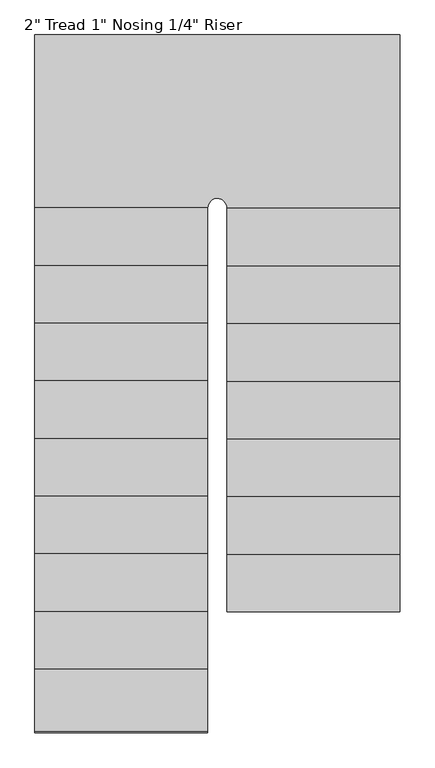
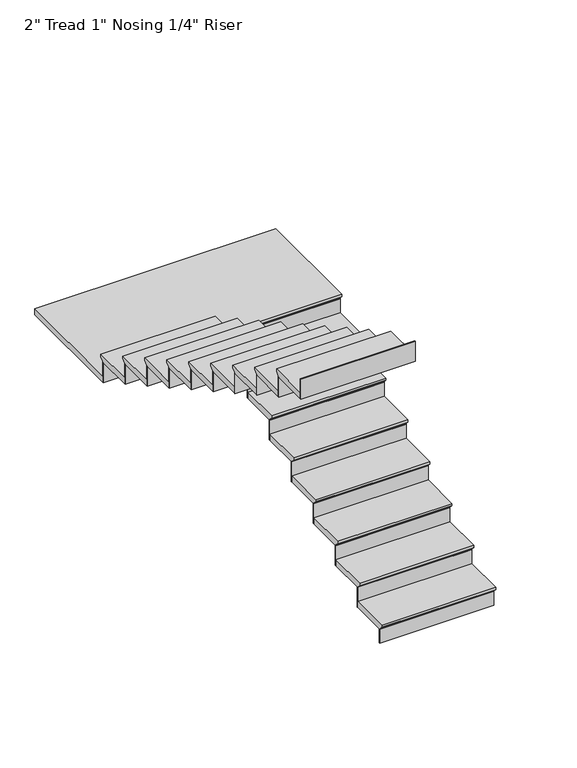
"""IFC4 building model written with IfcOpenShell, lengths in millimetres: stair flight geometry."""

from ifc_helpers import new_model, si_unit, frame, origin, place, context, project, spatial, polyline, circle_curve, ellipse_curve, faceted_brep, source, transform, mapped, element, save
from ifc_brep_helpers import plane_surface, revolved_surface, advanced_brep


def stair_flight_d4afe6aa(model_context):
    return source(origin(), model_context, "Body", "SolidModel", [
        faceted_brep([(-2547.8656154, 3686.6500875, 3198.2833333), (-2547.8656154, 3686.6500875, 3217.3333333), (-3462.2656154, 3686.6500875, 3217.3333333), (-3462.2656154, 3686.6500875, 3198.2833333), (-2547.8656154, 3712.0500875, 3172.8833333), (-3462.2656154, 3712.0500875, 3172.8833333), (-2547.8656154, 4016.8500875, 3217.3333333), (-3462.2656154, 4016.8500875, 3217.3333333), (-3462.2656154, 3712.0500875, 3166.5333333), (-3462.2656154, 4016.8500875, 3166.5333333), (-2547.8656154, 4016.8500875, 3166.5333333), (-2547.8656154, 3712.0500875, 3166.5333333)], [[[0, 1, 2, 3]], [[4, 0, 3, 5]], [[2, 1, 6, 7]], [[8, 9, 10, 11]], [[2, 7, 9, 8, 5, 3]], [[8, 11, 4, 5]], [[6, 1, 0, 4, 11, 10]], [[7, 6, 10, 9]]]),
        faceted_brep([(-2547.8656154, 3712.0500875, 3166.5333333), (-2547.8656154, 3712.0500875, 3048.0), (-2547.8656154, 3718.4000875, 3048.0), (-2547.8656154, 3718.4000875, 3166.5333333), (-3462.2656154, 3712.0500875, 3166.5333333), (-3462.2656154, 3718.4000875, 3166.5333333), (-3462.2656154, 3718.4000875, 3048.0), (-3462.2656154, 3712.0500875, 3048.0)], [[[0, 1, 2, 3]], [[4, 5, 6, 7]], [[1, 0, 4, 7]], [[2, 1, 7, 6]], [[3, 2, 6, 5]], [[0, 3, 5, 4]]]),
        faceted_brep([(-2547.8656154, 4016.8500875, 3335.8666667), (-2547.8656154, 4016.8500875, 3166.5333333), (-2547.8656154, 4023.2000875, 3166.5333333), (-2547.8656154, 4023.2000875, 3335.8666667), (-3462.2656154, 4016.8500875, 3335.8666667), (-3462.2656154, 4023.2000875, 3335.8666667), (-3462.2656154, 4023.2000875, 3166.5333333), (-3462.2656154, 4016.8500875, 3166.5333333)], [[[0, 1, 2, 3]], [[4, 5, 6, 7]], [[1, 0, 4, 7]], [[2, 1, 7, 6]], [[3, 2, 6, 5]], [[0, 3, 5, 4]]]),
        faceted_brep([(-3462.2656154, 3991.4500875, 3386.6666667), (-2547.8656154, 3991.4500875, 3386.6666667), (-2547.8656154, 4321.6500875, 3386.6666667), (-3462.2656154, 4321.6500875, 3386.6666667), (-3462.2656154, 4016.8500875, 3335.8666667), (-3462.2656154, 4321.6500875, 3335.8666667), (-2547.8656154, 4321.6500875, 3335.8666667), (-2547.8656154, 4016.8500875, 3335.8666667), (-3462.2656154, 4016.8500875, 3342.2166667), (-3462.2656154, 3991.4500875, 3367.6166667), (-2547.8656154, 4016.8500875, 3342.2166667), (-2547.8656154, 3991.4500875, 3367.6166667)], [[[0, 1, 2, 3]], [[4, 5, 6, 7]], [[0, 3, 5, 4, 8, 9]], [[4, 7, 10, 8]], [[2, 1, 11, 10, 7, 6]], [[3, 2, 6, 5]], [[11, 1, 0, 9]], [[10, 11, 9, 8]]]),
        faceted_brep([(-2547.8656154, 4321.6500875, 3505.2), (-2547.8656154, 4321.6500875, 3335.8666667), (-2547.8656154, 4328.0000875, 3335.8666667), (-2547.8656154, 4328.0000875, 3505.2), (-3462.2656154, 4321.6500875, 3505.2), (-3462.2656154, 4328.0000875, 3505.2), (-3462.2656154, 4328.0000875, 3335.8666667), (-3462.2656154, 4321.6500875, 3335.8666667)], [[[0, 1, 2, 3]], [[4, 5, 6, 7]], [[1, 0, 4, 7]], [[2, 1, 7, 6]], [[3, 2, 6, 5]], [[0, 3, 5, 4]]]),
        faceted_brep([(-3462.2656154, 4296.2500875, 3556.0), (-2547.8656154, 4296.2500875, 3556.0), (-2547.8656154, 4626.4500875, 3556.0), (-3462.2656154, 4626.4500875, 3556.0), (-3462.2656154, 4321.6500875, 3505.2), (-3462.2656154, 4626.4500875, 3505.2), (-2547.8656154, 4626.4500875, 3505.2), (-2547.8656154, 4321.6500875, 3505.2), (-3462.2656154, 4321.6500875, 3511.55), (-3462.2656154, 4296.2500875, 3536.95), (-2547.8656154, 4321.6500875, 3511.55), (-2547.8656154, 4296.2500875, 3536.95)], [[[0, 1, 2, 3]], [[4, 5, 6, 7]], [[0, 3, 5, 4, 8, 9]], [[4, 7, 10, 8]], [[2, 1, 11, 10, 7, 6]], [[3, 2, 6, 5]], [[11, 1, 0, 9]], [[10, 11, 9, 8]]]),
        faceted_brep([(-2547.8656154, 4626.4500875, 3674.5333333), (-2547.8656154, 4626.4500875, 3505.2), (-2547.8656154, 4632.8000875, 3505.2), (-2547.8656154, 4632.8000875, 3674.5333333), (-3462.2656154, 4626.4500875, 3674.5333333), (-3462.2656154, 4632.8000875, 3674.5333333), (-3462.2656154, 4632.8000875, 3505.2), (-3462.2656154, 4626.4500875, 3505.2)], [[[0, 1, 2, 3]], [[4, 5, 6, 7]], [[1, 0, 4, 7]], [[2, 1, 7, 6]], [[3, 2, 6, 5]], [[0, 3, 5, 4]]]),
        faceted_brep([(-3462.2656154, 4601.0500875, 3725.3333333), (-2547.8656154, 4601.0500875, 3725.3333333), (-2547.8656154, 4931.2500875, 3725.3333333), (-3462.2656154, 4931.2500875, 3725.3333333), (-3462.2656154, 4626.4500875, 3674.5333333), (-3462.2656154, 4931.2500875, 3674.5333333), (-2547.8656154, 4931.2500875, 3674.5333333), (-2547.8656154, 4626.4500875, 3674.5333333), (-3462.2656154, 4626.4500875, 3680.8833333), (-3462.2656154, 4601.0500875, 3706.2833333), (-2547.8656154, 4626.4500875, 3680.8833333), (-2547.8656154, 4601.0500875, 3706.2833333)], [[[0, 1, 2, 3]], [[4, 5, 6, 7]], [[0, 3, 5, 4, 8, 9]], [[4, 7, 10, 8]], [[2, 1, 11, 10, 7, 6]], [[3, 2, 6, 5]], [[11, 1, 0, 9]], [[10, 11, 9, 8]]]),
        faceted_brep([(-2547.8656154, 4931.2500875, 3843.8666667), (-2547.8656154, 4931.2500875, 3674.5333333), (-2547.8656154, 4937.6000875, 3674.5333333), (-2547.8656154, 4937.6000875, 3843.8666667), (-3462.2656154, 4931.2500875, 3843.8666667), (-3462.2656154, 4937.6000875, 3843.8666667), (-3462.2656154, 4937.6000875, 3674.5333333), (-3462.2656154, 4931.2500875, 3674.5333333)], [[[0, 1, 2, 3]], [[4, 5, 6, 7]], [[1, 0, 4, 7]], [[2, 1, 7, 6]], [[3, 2, 6, 5]], [[0, 3, 5, 4]]]),
        faceted_brep([(-3462.2656154, 4905.8500875, 3894.6666667), (-2547.8656154, 4905.8500875, 3894.6666667), (-2547.8656154, 5236.0500875, 3894.6666667), (-3462.2656154, 5236.0500875, 3894.6666667), (-3462.2656154, 4931.2500875, 3843.8666667), (-3462.2656154, 5236.0500875, 3843.8666667), (-2547.8656154, 5236.0500875, 3843.8666667), (-2547.8656154, 4931.2500875, 3843.8666667), (-3462.2656154, 4931.2500875, 3850.2166667), (-3462.2656154, 4905.8500875, 3875.6166667), (-2547.8656154, 4931.2500875, 3850.2166667), (-2547.8656154, 4905.8500875, 3875.6166667)], [[[0, 1, 2, 3]], [[4, 5, 6, 7]], [[0, 3, 5, 4, 8, 9]], [[4, 7, 10, 8]], [[2, 1, 11, 10, 7, 6]], [[3, 2, 6, 5]], [[11, 1, 0, 9]], [[10, 11, 9, 8]]]),
        faceted_brep([(-2547.8656154, 5236.0500875, 4013.2), (-2547.8656154, 5236.0500875, 3843.8666667), (-2547.8656154, 5242.4000875, 3843.8666667), (-2547.8656154, 5242.4000875, 4013.2), (-3462.2656154, 5236.0500875, 4013.2), (-3462.2656154, 5242.4000875, 4013.2), (-3462.2656154, 5242.4000875, 3843.8666667), (-3462.2656154, 5236.0500875, 3843.8666667)], [[[0, 1, 2, 3]], [[4, 5, 6, 7]], [[1, 0, 4, 7]], [[2, 1, 7, 6]], [[3, 2, 6, 5]], [[0, 3, 5, 4]]]),
        faceted_brep([(-3462.2656154, 5210.6500875, 4064.0), (-2547.8656154, 5210.6500875, 4064.0), (-2547.8656154, 5540.8500875, 4064.0), (-3462.2656154, 5540.8500875, 4064.0), (-3462.2656154, 5236.0500875, 4013.2), (-3462.2656154, 5540.8500875, 4013.2), (-2547.8656154, 5540.8500875, 4013.2), (-2547.8656154, 5236.0500875, 4013.2), (-3462.2656154, 5236.0500875, 4019.55), (-3462.2656154, 5210.6500875, 4044.95), (-2547.8656154, 5236.0500875, 4019.55), (-2547.8656154, 5210.6500875, 4044.95)], [[[0, 1, 2, 3]], [[4, 5, 6, 7]], [[0, 3, 5, 4, 8, 9]], [[4, 7, 10, 8]], [[2, 1, 11, 10, 7, 6]], [[3, 2, 6, 5]], [[11, 1, 0, 9]], [[10, 11, 9, 8]]]),
        faceted_brep([(-2547.8656154, 5540.8500875, 4182.5333333), (-2547.8656154, 5540.8500875, 4013.2), (-2547.8656154, 5547.2000875, 4013.2), (-2547.8656154, 5547.2000875, 4182.5333333), (-3462.2656154, 5540.8500875, 4182.5333333), (-3462.2656154, 5547.2000875, 4182.5333333), (-3462.2656154, 5547.2000875, 4013.2), (-3462.2656154, 5540.8500875, 4013.2)], [[[0, 1, 2, 3]], [[4, 5, 6, 7]], [[1, 0, 4, 7]], [[2, 1, 7, 6]], [[3, 2, 6, 5]], [[0, 3, 5, 4]]]),
        faceted_brep([(-3462.2656154, 5515.4500875, 4233.3333333), (-2547.8656154, 5515.4500875, 4233.3333333), (-2547.8656154, 5845.6500875, 4233.3333333), (-3462.2656154, 5845.6500875, 4233.3333333), (-3462.2656154, 5540.8500875, 4182.5333333), (-3462.2656154, 5845.6500875, 4182.5333333), (-2547.8656154, 5845.6500875, 4182.5333333), (-2547.8656154, 5540.8500875, 4182.5333333), (-3462.2656154, 5540.8500875, 4188.8833333), (-3462.2656154, 5515.4500875, 4214.2833333), (-2547.8656154, 5540.8500875, 4188.8833333), (-2547.8656154, 5515.4500875, 4214.2833333)], [[[0, 1, 2, 3]], [[4, 5, 6, 7]], [[0, 3, 5, 4, 8, 9]], [[4, 7, 10, 8]], [[2, 1, 11, 10, 7, 6]], [[3, 2, 6, 5]], [[11, 1, 0, 9]], [[10, 11, 9, 8]]]),
        advanced_brep(
        [(-2547.8656154, 5845.6500875, 4351.8666667), (-2547.8656154, 5845.6500875, 4182.5333333), (-2547.8656154, 5852.0000875, 4182.5333333), (-2547.8656154, 5852.0000875, 4351.8666667), (-3469.0715249, 5845.6500875, 4351.8666667), (-3473.4098781, 5852.0000875, 4351.8666667), (-3473.4098781, 5852.0000875, 4182.5333333), (-3469.0715249, 5845.6500875, 4182.5333333)],
        [
            (0, 1),
            (1, 2),
            (2, 3),
            (3, 0),
            (4, 5, circle_curve(frame((-3513.0656154, 5820.2500875, 4351.8666667), z_axis=(0.0, 0.0, 1.0), x_axis=(1.0, 0.0, 0.0)), 50.8)),
            (5, 6),
            (6, 7, circle_curve(frame((-3513.0656154, 5820.2500875, 4182.5333333), z_axis=(0.0, 0.0, -1.0), x_axis=(1.0, 0.0, 0.0)), 50.8)),
            (7, 4),
            (0, 4),
            (7, 1),
            (6, 2),
            (5, 3),
        ],
        [
            plane_surface(frame((-2547.8656154, 5845.6500875, 4402.6666667), z_axis=(1.0, 0.0, 0.0), x_axis=(0.0, 1.0, 0.0))),
            revolved_surface(polyline([(-3462.2656153999997, 5820.2500875, 4182.5333333), (-3462.2656153999997, 5820.2500875, 4351.8666667)]), (-3513.0656154, 5820.2500875, 4351.8666667), (0.0, 0.0, -1.0)),
            plane_surface(frame((-2547.8656154, 5845.6500875, 4351.8666667), z_axis=(0.0, -1.0, 0.0), x_axis=(-1.0, 0.0, 0.0))),
            plane_surface(frame((-2547.8656154, 5845.6500875, 4182.5333333), z_axis=(0.0, 0.0, -1.0), x_axis=(-1.0, 0.0, 0.0))),
            plane_surface(frame((-2547.8656154, 5852.0000875, 4182.5333333), z_axis=(0.0, 1.0, 0.0), x_axis=(-1.0, 0.0, 0.0))),
            plane_surface(frame((-2547.8656154, 5852.0000875, 4351.8666667), z_axis=(0.0, 0.0, 1.0), x_axis=(-1.0, 0.0, 0.0))),
        ],
        [
            (0, [[1, 2, 3, 4]]),
            (1, [[5, 6, 7, 8]]),
            (2, [[-1, 9, -8, 10]]),
            (3, [[-2, -10, -7, 11]]),
            (4, [[-3, -11, -6, 12]]),
            (5, [[-4, -12, -5, -9]]),
        ],
    ),
        advanced_brep(
        [(-3563.8656154, 5794.8500875, 4402.6666667), (-3563.8656154, 5820.2500875, 4402.6666667), (-3469.0715249, 5845.6500875, 4402.6666667), (-3462.2656154, 5820.2500875, 4402.6666667), (-2547.8656154, 5820.2500875, 4402.6666667), (-2547.8656154, 6734.6500875, 4402.6666667), (-4478.2656154, 6734.6500875, 4402.6666667), (-4478.2656154, 5794.8500875, 4402.6666667), (-3563.8656154, 5820.2500875, 4351.8666667), (-3563.8656154, 5794.8500875, 4351.8666667), (-4478.2656154, 5794.8500875, 4351.8666667), (-4478.2656154, 6734.6500875, 4351.8666667), (-2547.8656154, 6734.6500875, 4351.8666667), (-2547.8656154, 5845.6500875, 4351.8666667), (-3469.0715249, 5845.6500875, 4351.8666667), (-3469.0715249, 5845.6500875, 4358.2166667), (-2547.8656154, 5845.6500875, 4358.2166667), (-2547.8656154, 5820.2500875, 4383.6166667), (-3462.2656154, 5820.2500875, 4383.6166667)],
        [
            (0, 1),
            (1, 2, circle_curve(frame((-3513.0656154, 5820.2500875, 4402.6666667), z_axis=(0.0, 0.0, -1.0), x_axis=(1.0, 0.0, 0.0)), 50.8)),
            (2, 3, circle_curve(frame((-3513.0656154, 5820.2500875, 4402.6666667), z_axis=(0.0, 0.0, -1.0), x_axis=(1.0, 0.0, 0.0)), 50.8)),
            (3, 4),
            (4, 5),
            (5, 6),
            (6, 7),
            (7, 0),
            (8, 9),
            (9, 10),
            (10, 11),
            (11, 12),
            (12, 13),
            (13, 14),
            (14, 8, circle_curve(frame((-3513.0656154, 5820.2500875, 4351.8666667), z_axis=(0.0, 0.0, 1.0), x_axis=(1.0, 0.0, 0.0)), 50.8)),
            (0, 9),
            (8, 1),
            (14, 15),
            (15, 2),
            (13, 16),
            (16, 15),
            (4, 17),
            (17, 16),
            (12, 5),
            (11, 6),
            (10, 7),
            (18, 3),
            (15, 18, ellipse_curve(frame((-3513.0656154, 5820.2500875, 4383.6166667), z_axis=(0.0, -0.7071067811865489, -0.7071067811865461), x_axis=(0.0, 0.7071067811865461, -0.7071067811865489)), 71.842049, 50.8)),
            (18, 17),
        ],
        [
            plane_surface(frame((-3563.8656154, 5820.2500875, 4402.6666667), z_axis=(0.0, 0.0, 1.0), x_axis=(0.0, 1.0, 0.0))),
            plane_surface(frame((-3563.8656154, 5820.2500875, 4351.8666667), z_axis=(0.0, 0.0, -1.0), x_axis=(0.0, -1.0, 0.0))),
            plane_surface(frame((-3563.8656154, 5794.8500875, 4402.6666667), z_axis=(1.0, 0.0, 0.0), x_axis=(0.0, 0.0, -1.0))),
            revolved_surface(polyline([(-3462.2656153999997, 5820.2500875, 4351.8666667), (-3462.2656153999997, 5820.2500875, 4402.6666667)]), (-3513.0656154, 5820.2500875, 4351.8666667), (0.0, 0.0, -1.0)),
            plane_surface(frame((-3469.0715249, 5845.6500875, 4402.6666667), z_axis=(0.0, -1.0, 0.0), x_axis=(0.0, 0.0, -1.0))),
            plane_surface(frame((-2547.8656154, 5845.6500875, 4402.6666667), z_axis=(1.0, 0.0, 0.0), x_axis=(0.0, 0.0, -1.0))),
            plane_surface(frame((-2547.8656154, 6734.6500875, 4402.6666667), z_axis=(0.0, 1.0, 0.0), x_axis=(0.0, 0.0, -1.0))),
            plane_surface(frame((-4478.2656154, 6734.6500875, 4402.6666667), z_axis=(-1.0, 0.0, 0.0), x_axis=(0.0, 0.0, -1.0))),
            plane_surface(frame((-4478.2656154, 5794.8500875, 4402.6666667), z_axis=(0.0, -1.0, 0.0), x_axis=(0.0, 0.0, -1.0))),
            revolved_surface(polyline([(-3462.2656153999997, 5820.2500875, 4332.816666677763), (-3462.2656153999997, 5820.2500875, 4434.416666722236)]), (-3513.0656154, 5820.2500875, 4351.8666667), (0.0, 0.0, -1.0)),
            plane_surface(frame((-2547.8656154, 5820.2500875, 4402.6666667), z_axis=(0.0, -1.0, 0.0), x_axis=(-1.0, 0.0, 0.0))),
            plane_surface(frame((-2547.8656154, 5820.2500875, 4383.6166667), z_axis=(0.0, -0.7071067811865489, -0.7071067811865461), x_axis=(-1.0, 0.0, 0.0))),
        ],
        [
            (0, [[1, 2, 3, 4, 5, 6, 7, 8]]),
            (1, [[9, 10, 11, 12, 13, 14, 15]]),
            (2, [[-1, 16, -9, 17]]),
            (3, [[-2, -17, -15, 18, 19]]),
            (4, [[-14, 20, 21, -18]]),
            (5, [[-5, 22, 23, -20, -13, 24]]),
            (6, [[-6, -24, -12, 25]]),
            (7, [[-7, -25, -11, 26]]),
            (8, [[-8, -26, -10, -16]]),
            (9, [[27, -3, -19, 28]]),
            (10, [[-22, -4, -27, 29]]),
            (11, [[-23, -29, -28, -21]]),
        ],
    ),
        faceted_brep([(-4478.2656154, 5794.8500875, 4521.2), (-4478.2656154, 5794.8500875, 4351.8666667), (-4478.2656154, 5788.5000875, 4351.8666667), (-4478.2656154, 5788.5000875, 4521.2), (-3563.8656154, 5794.8500875, 4521.2), (-3563.8656154, 5788.5000875, 4521.2), (-3563.8656154, 5788.5000875, 4351.8666667), (-3563.8656154, 5794.8500875, 4351.8666667)], [[[0, 1, 2, 3]], [[4, 5, 6, 7]], [[1, 0, 4, 7]], [[2, 1, 7, 6]], [[3, 2, 6, 5]], [[0, 3, 5, 4]]]),
        faceted_brep([(-3563.8656154, 5820.2500875, 4572.0), (-4478.2656154, 5820.2500875, 4572.0), (-4478.2656154, 5490.0500875, 4572.0), (-3563.8656154, 5490.0500875, 4572.0), (-3563.8656154, 5794.8500875, 4521.2), (-3563.8656154, 5490.0500875, 4521.2), (-4478.2656154, 5490.0500875, 4521.2), (-4478.2656154, 5794.8500875, 4521.2), (-3563.8656154, 5794.8500875, 4527.55), (-3563.8656154, 5820.2500875, 4552.95), (-4478.2656154, 5794.8500875, 4527.55), (-4478.2656154, 5820.2500875, 4552.95)], [[[0, 1, 2, 3]], [[4, 5, 6, 7]], [[0, 3, 5, 4, 8, 9]], [[4, 7, 10, 8]], [[2, 1, 11, 10, 7, 6]], [[3, 2, 6, 5]], [[11, 1, 0, 9]], [[10, 11, 9, 8]]]),
        faceted_brep([(-4478.2656154, 5490.0500875, 4690.5333333), (-4478.2656154, 5490.0500875, 4521.2), (-4478.2656154, 5483.7000875, 4521.2), (-4478.2656154, 5483.7000875, 4690.5333333), (-3563.8656154, 5490.0500875, 4690.5333333), (-3563.8656154, 5483.7000875, 4690.5333333), (-3563.8656154, 5483.7000875, 4521.2), (-3563.8656154, 5490.0500875, 4521.2)], [[[0, 1, 2, 3]], [[4, 5, 6, 7]], [[1, 0, 4, 7]], [[2, 1, 7, 6]], [[3, 2, 6, 5]], [[0, 3, 5, 4]]]),
        faceted_brep([(-3563.8656154, 5515.4500875, 4741.3333333), (-4478.2656154, 5515.4500875, 4741.3333333), (-4478.2656154, 5185.2500875, 4741.3333333), (-3563.8656154, 5185.2500875, 4741.3333333), (-3563.8656154, 5490.0500875, 4690.5333333), (-3563.8656154, 5185.2500875, 4690.5333333), (-4478.2656154, 5185.2500875, 4690.5333333), (-4478.2656154, 5490.0500875, 4690.5333333), (-3563.8656154, 5490.0500875, 4696.8833333), (-3563.8656154, 5515.4500875, 4722.2833333), (-4478.2656154, 5490.0500875, 4696.8833333), (-4478.2656154, 5515.4500875, 4722.2833333)], [[[0, 1, 2, 3]], [[4, 5, 6, 7]], [[0, 3, 5, 4, 8, 9]], [[4, 7, 10, 8]], [[2, 1, 11, 10, 7, 6]], [[3, 2, 6, 5]], [[11, 1, 0, 9]], [[10, 11, 9, 8]]]),
        faceted_brep([(-4478.2656154, 5185.2500875, 4859.8666667), (-4478.2656154, 5185.2500875, 4690.5333333), (-4478.2656154, 5178.9000875, 4690.5333333), (-4478.2656154, 5178.9000875, 4859.8666667), (-3563.8656154, 5185.2500875, 4859.8666667), (-3563.8656154, 5178.9000875, 4859.8666667), (-3563.8656154, 5178.9000875, 4690.5333333), (-3563.8656154, 5185.2500875, 4690.5333333)], [[[0, 1, 2, 3]], [[4, 5, 6, 7]], [[1, 0, 4, 7]], [[2, 1, 7, 6]], [[3, 2, 6, 5]], [[0, 3, 5, 4]]]),
        faceted_brep([(-3563.8656154, 5210.6500875, 4910.6666667), (-4478.2656154, 5210.6500875, 4910.6666667), (-4478.2656154, 4880.4500875, 4910.6666667), (-3563.8656154, 4880.4500875, 4910.6666667), (-3563.8656154, 5185.2500875, 4859.8666667), (-3563.8656154, 4880.4500875, 4859.8666667), (-4478.2656154, 4880.4500875, 4859.8666667), (-4478.2656154, 5185.2500875, 4859.8666667), (-3563.8656154, 5185.2500875, 4866.2166667), (-3563.8656154, 5210.6500875, 4891.6166667), (-4478.2656154, 5185.2500875, 4866.2166667), (-4478.2656154, 5210.6500875, 4891.6166667)], [[[0, 1, 2, 3]], [[4, 5, 6, 7]], [[0, 3, 5, 4, 8, 9]], [[4, 7, 10, 8]], [[2, 1, 11, 10, 7, 6]], [[3, 2, 6, 5]], [[11, 1, 0, 9]], [[10, 11, 9, 8]]]),
        faceted_brep([(-4478.2656154, 4880.4500875, 5029.2), (-4478.2656154, 4880.4500875, 4859.8666667), (-4478.2656154, 4874.1000875, 4859.8666667), (-4478.2656154, 4874.1000875, 5029.2), (-3563.8656154, 4880.4500875, 5029.2), (-3563.8656154, 4874.1000875, 5029.2), (-3563.8656154, 4874.1000875, 4859.8666667), (-3563.8656154, 4880.4500875, 4859.8666667)], [[[0, 1, 2, 3]], [[4, 5, 6, 7]], [[1, 0, 4, 7]], [[2, 1, 7, 6]], [[3, 2, 6, 5]], [[0, 3, 5, 4]]]),
        faceted_brep([(-3563.8656154, 4905.8500875, 5080.0), (-4478.2656154, 4905.8500875, 5080.0), (-4478.2656154, 4575.6500875, 5080.0), (-3563.8656154, 4575.6500875, 5080.0), (-3563.8656154, 4880.4500875, 5029.2), (-3563.8656154, 4575.6500875, 5029.2), (-4478.2656154, 4575.6500875, 5029.2), (-4478.2656154, 4880.4500875, 5029.2), (-3563.8656154, 4880.4500875, 5035.55), (-3563.8656154, 4905.8500875, 5060.95), (-4478.2656154, 4880.4500875, 5035.55), (-4478.2656154, 4905.8500875, 5060.95)], [[[0, 1, 2, 3]], [[4, 5, 6, 7]], [[0, 3, 5, 4, 8, 9]], [[4, 7, 10, 8]], [[2, 1, 11, 10, 7, 6]], [[3, 2, 6, 5]], [[11, 1, 0, 9]], [[10, 11, 9, 8]]]),
        faceted_brep([(-4478.2656154, 4575.6500875, 5198.5333333), (-4478.2656154, 4575.6500875, 5029.2), (-4478.2656154, 4569.3000875, 5029.2), (-4478.2656154, 4569.3000875, 5198.5333333), (-3563.8656154, 4575.6500875, 5198.5333333), (-3563.8656154, 4569.3000875, 5198.5333333), (-3563.8656154, 4569.3000875, 5029.2), (-3563.8656154, 4575.6500875, 5029.2)], [[[0, 1, 2, 3]], [[4, 5, 6, 7]], [[1, 0, 4, 7]], [[2, 1, 7, 6]], [[3, 2, 6, 5]], [[0, 3, 5, 4]]]),
        faceted_brep([(-3563.8656154, 4601.0500875, 5249.3333333), (-4478.2656154, 4601.0500875, 5249.3333333), (-4478.2656154, 4270.8500875, 5249.3333333), (-3563.8656154, 4270.8500875, 5249.3333333), (-3563.8656154, 4575.6500875, 5198.5333333), (-3563.8656154, 4270.8500875, 5198.5333333), (-4478.2656154, 4270.8500875, 5198.5333333), (-4478.2656154, 4575.6500875, 5198.5333333), (-3563.8656154, 4575.6500875, 5204.8833333), (-3563.8656154, 4601.0500875, 5230.2833333), (-4478.2656154, 4575.6500875, 5204.8833333), (-4478.2656154, 4601.0500875, 5230.2833333)], [[[0, 1, 2, 3]], [[4, 5, 6, 7]], [[0, 3, 5, 4, 8, 9]], [[4, 7, 10, 8]], [[2, 1, 11, 10, 7, 6]], [[3, 2, 6, 5]], [[11, 1, 0, 9]], [[10, 11, 9, 8]]]),
        faceted_brep([(-4478.2656154, 4270.8500875, 5367.8666667), (-4478.2656154, 4270.8500875, 5198.5333333), (-4478.2656154, 4264.5000875, 5198.5333333), (-4478.2656154, 4264.5000875, 5367.8666667), (-3563.8656154, 4270.8500875, 5367.8666667), (-3563.8656154, 4264.5000875, 5367.8666667), (-3563.8656154, 4264.5000875, 5198.5333333), (-3563.8656154, 4270.8500875, 5198.5333333)], [[[0, 1, 2, 3]], [[4, 5, 6, 7]], [[1, 0, 4, 7]], [[2, 1, 7, 6]], [[3, 2, 6, 5]], [[0, 3, 5, 4]]]),
        faceted_brep([(-3563.8656154, 4296.2500875, 5418.6666667), (-4478.2656154, 4296.2500875, 5418.6666667), (-4478.2656154, 3966.0500875, 5418.6666667), (-3563.8656154, 3966.0500875, 5418.6666667), (-3563.8656154, 4270.8500875, 5367.8666667), (-3563.8656154, 3966.0500875, 5367.8666667), (-4478.2656154, 3966.0500875, 5367.8666667), (-4478.2656154, 4270.8500875, 5367.8666667), (-3563.8656154, 4270.8500875, 5374.2166667), (-3563.8656154, 4296.2500875, 5399.6166667), (-4478.2656154, 4270.8500875, 5374.2166667), (-4478.2656154, 4296.2500875, 5399.6166667)], [[[0, 1, 2, 3]], [[4, 5, 6, 7]], [[0, 3, 5, 4, 8, 9]], [[4, 7, 10, 8]], [[2, 1, 11, 10, 7, 6]], [[3, 2, 6, 5]], [[11, 1, 0, 9]], [[10, 11, 9, 8]]]),
        faceted_brep([(-4478.2656154, 3966.0500875, 5537.2), (-4478.2656154, 3966.0500875, 5367.8666667), (-4478.2656154, 3959.7000875, 5367.8666667), (-4478.2656154, 3959.7000875, 5537.2), (-3563.8656154, 3966.0500875, 5537.2), (-3563.8656154, 3959.7000875, 5537.2), (-3563.8656154, 3959.7000875, 5367.8666667), (-3563.8656154, 3966.0500875, 5367.8666667)], [[[0, 1, 2, 3]], [[4, 5, 6, 7]], [[1, 0, 4, 7]], [[2, 1, 7, 6]], [[3, 2, 6, 5]], [[0, 3, 5, 4]]]),
        faceted_brep([(-3563.8656154, 3991.4500875, 5588.0), (-4478.2656154, 3991.4500875, 5588.0), (-4478.2656154, 3661.2500875, 5588.0), (-3563.8656154, 3661.2500875, 5588.0), (-3563.8656154, 3966.0500875, 5537.2), (-3563.8656154, 3661.2500875, 5537.2), (-4478.2656154, 3661.2500875, 5537.2), (-4478.2656154, 3966.0500875, 5537.2), (-3563.8656154, 3966.0500875, 5543.55), (-3563.8656154, 3991.4500875, 5568.95), (-4478.2656154, 3966.0500875, 5543.55), (-4478.2656154, 3991.4500875, 5568.95)], [[[0, 1, 2, 3]], [[4, 5, 6, 7]], [[0, 3, 5, 4, 8, 9]], [[4, 7, 10, 8]], [[2, 1, 11, 10, 7, 6]], [[3, 2, 6, 5]], [[11, 1, 0, 9]], [[10, 11, 9, 8]]]),
        faceted_brep([(-4478.2656154, 3661.2500875, 5706.5333333), (-4478.2656154, 3661.2500875, 5537.2), (-4478.2656154, 3654.9000875, 5537.2), (-4478.2656154, 3654.9000875, 5706.5333333), (-3563.8656154, 3661.2500875, 5706.5333333), (-3563.8656154, 3654.9000875, 5706.5333333), (-3563.8656154, 3654.9000875, 5537.2), (-3563.8656154, 3661.2500875, 5537.2)], [[[0, 1, 2, 3]], [[4, 5, 6, 7]], [[1, 0, 4, 7]], [[2, 1, 7, 6]], [[3, 2, 6, 5]], [[0, 3, 5, 4]]]),
        faceted_brep([(-3563.8656154, 3686.6500875, 5757.3333333), (-4478.2656154, 3686.6500875, 5757.3333333), (-4478.2656154, 3356.4500875, 5757.3333333), (-3563.8656154, 3356.4500875, 5757.3333333), (-3563.8656154, 3661.2500875, 5706.5333333), (-3563.8656154, 3356.4500875, 5706.5333333), (-4478.2656154, 3356.4500875, 5706.5333333), (-4478.2656154, 3661.2500875, 5706.5333333), (-3563.8656154, 3661.2500875, 5712.8833333), (-3563.8656154, 3686.6500875, 5738.2833333), (-4478.2656154, 3661.2500875, 5712.8833333), (-4478.2656154, 3686.6500875, 5738.2833333)], [[[0, 1, 2, 3]], [[4, 5, 6, 7]], [[0, 3, 5, 4, 8, 9]], [[4, 7, 10, 8]], [[2, 1, 11, 10, 7, 6]], [[3, 2, 6, 5]], [[11, 1, 0, 9]], [[10, 11, 9, 8]]]),
        faceted_brep([(-4478.2656154, 3356.4500875, 5875.8666667), (-4478.2656154, 3356.4500875, 5706.5333333), (-4478.2656154, 3350.1000875, 5706.5333333), (-4478.2656154, 3350.1000875, 5875.8666667), (-3563.8656154, 3356.4500875, 5875.8666667), (-3563.8656154, 3350.1000875, 5875.8666667), (-3563.8656154, 3350.1000875, 5706.5333333), (-3563.8656154, 3356.4500875, 5706.5333333)], [[[0, 1, 2, 3]], [[4, 5, 6, 7]], [[1, 0, 4, 7]], [[2, 1, 7, 6]], [[3, 2, 6, 5]], [[0, 3, 5, 4]]]),
        faceted_brep([(-4478.2656154, 3051.6500875, 6045.2), (-4478.2656154, 3051.6500875, 5875.8666667), (-4478.2656154, 3045.3000875, 5875.8666667), (-4478.2656154, 3045.3000875, 6045.2), (-3563.8656154, 3051.6500875, 6045.2), (-3563.8656154, 3045.3000875, 6045.2), (-3563.8656154, 3045.3000875, 5875.8666667), (-3563.8656154, 3051.6500875, 5875.8666667)], [[[0, 1, 2, 3]], [[4, 5, 6, 7]], [[1, 0, 4, 7]], [[2, 1, 7, 6]], [[3, 2, 6, 5]], [[0, 3, 5, 4]]]),
        faceted_brep([(-3563.8656154, 3381.8500875, 5926.6666667), (-4478.2656154, 3381.8500875, 5926.6666667), (-4478.2656154, 3051.6500875, 5926.6666667), (-3563.8656154, 3051.6500875, 5926.6666667), (-3563.8656154, 3356.4500875, 5875.8666667), (-3563.8656154, 3051.6500875, 5875.8666667), (-4478.2656154, 3051.6500875, 5875.8666667), (-4478.2656154, 3356.4500875, 5875.8666667), (-3563.8656154, 3356.4500875, 5882.2166667), (-3563.8656154, 3381.8500875, 5907.6166667), (-4478.2656154, 3356.4500875, 5882.2166667), (-4478.2656154, 3381.8500875, 5907.6166667)], [[[0, 1, 2, 3]], [[4, 5, 6, 7]], [[0, 3, 5, 4, 8, 9]], [[4, 7, 10, 8]], [[2, 1, 11, 10, 7, 6]], [[3, 2, 6, 5]], [[11, 1, 0, 9]], [[10, 11, 9, 8]]]),
    ])


if __name__ == "__main__":
    model = new_model("IFC4")
    model_context = context("Model", 3, world=origin())
    ifc_project = project(units=[si_unit("LENGTHUNIT", "METRE", prefix="MILLI")], contexts=[model_context])
    site = spatial("IfcSite", under=ifc_project)
    building = spatial("IfcBuilding", under=site)
    placement = place(None, origin())
    stair_flight_shape = stair_flight_d4afe6aa(model_context)
    element("IfcStairFlight", 1, ObjectType="2\" Tread 1\" Nosing 1/4\" Riser", at=placement, inside=building, context=model_context, shape_type="MappedRepresentation", body=[
        mapped(stair_flight_shape, transform((0.0, 0.0, 0.0), x_axis=(1.0, 0.0, 0.0), y_axis=(0.0, 1.0, 0.0), z_axis=(0.0, 0.0, 1.0))),
    ])
    save(model, "model.ifc")
